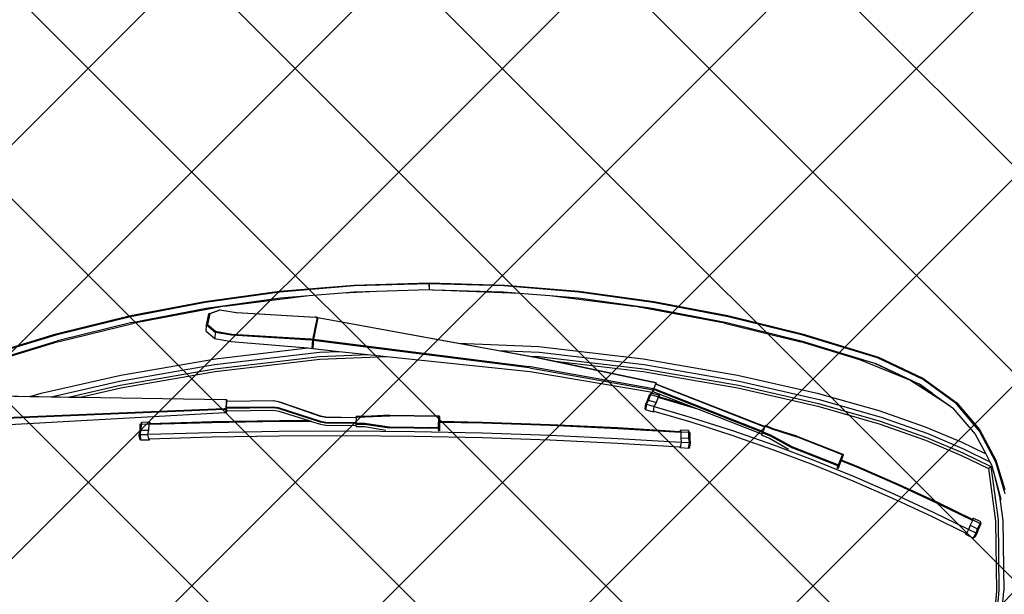
# Model space of a CAD drawing. Units: inches. Extents: x 2167 to 2589, y 1680 to 2489.
# Tile 26 of 38: x 2356 to 2389, y 1796 to 1815. Entities that reach past the tile are written whole.
import ezdxf

# ---------------------------------------------------------------- set-up
doc = ezdxf.new("R2010")
doc.units = ezdxf.units.IN
doc.header["$MEASUREMENT"] = 0
doc.layers.get('0').update_dxf_attribs({"color": 250})
doc.layers.add('C-PRKG-VEHS', color=8, linetype='Continuous', lineweight=13)
doc.layers.add('L-PVMT-PATT', color=252, linetype='Continuous', lineweight=13)
doc.layers.add('Edges', color=250, linetype='Continuous')

# ---------------------------------------------------------------- blocks, each defined once
blk = doc.blocks.new('Nissan Qashqai pl')
at = {"layer": 'Edges'}
for p, q in [((8.4814, 12.6029), (8.5166, 12.6135)), ((8.5216, 12.6139), (8.4838, 12.6027)), ((8.5538, 12.6111), (8.6387, 12.6123)), ((8.6721, 12.6093), (8.6387, 12.6123)), ((8.4444, 12.5834), (8.4814, 12.6029)), ((8.4838, 12.6027), (8.4462, 12.5833)), ((8.4867, 12.5977), (8.5039, 12.6023)), ((8.4889, 12.5969), (8.5531, 12.6055)), ((8.4914, 12.5942), (8.5544, 12.6026)), ((8.5039, 12.6023), (8.528, 12.6088)), ((8.5216, 12.6068), (8.5039, 12.6023)), ((8.5216, 12.6068), (8.5538, 12.6111)), ((8.5301, 12.609), (8.5216, 12.6068)), ((8.5531, 12.6055), (8.6375, 12.6066)), ((8.5544, 12.6026), (8.6386, 12.6037)), ((8.6375, 12.6066), (8.7481, 12.5968)), ((8.6386, 12.6037), (8.7491, 12.594)), ((8.4499, 12.5782), (8.4737, 12.5908)), ((8.4594, 12.5611), (8.4737, 12.5908)), ((8.468, 12.5648), (8.4831, 12.5957)), ((8.4725, 12.563), (8.4889, 12.5969)), ((8.4737, 12.5908), (8.4831, 12.5957)), ((8.4756, 12.5615), (8.4914, 12.5942)), ((8.4831, 12.5957), (8.4867, 12.5977)), ((8.4914, 12.5942), (8.4889, 12.5969)), ((8.4122, 12.5558), (8.4444, 12.5834)), ((8.4462, 12.5833), (8.4134, 12.5554)), ((8.4183, 12.5508), (8.4499, 12.5782)), ((8.5554, 12.5847), (8.551, 12.5757)), ((8.5529, 12.5751), (8.5572, 12.5841)), ((8.5574, 12.5849), (8.5554, 12.5847)), ((8.5572, 12.5841), (8.5554, 12.5847)), ((8.5639, 12.581), (8.5572, 12.5841)), ((8.5574, 12.5849), (8.5584, 12.5846)), ((8.5582, 12.5845), (8.5574, 12.5849)), ((8.5584, 12.5846), (8.5649, 12.5816)), ((8.5595, 12.572), (8.5639, 12.581)), ((8.5687, 12.5791), (8.5639, 12.581)), ((8.5644, 12.5701), (8.5687, 12.5791)), ((8.5649, 12.5816), (8.5693, 12.5799)), ((8.5687, 12.5791), (8.5693, 12.5799)), ((8.5749, 12.5757), (8.5687, 12.5791)), ((8.5693, 12.5799), (8.5739, 12.5774)), ((8.5739, 12.5774), (8.5749, 12.5757)), ((8.4493, 12.5212), (8.468, 12.5648)), ((8.5527, 12.5749), (8.5323, 12.5332)), ((8.5537, 12.5747), (8.5332, 12.5329)), ((8.5647, 12.57), (8.5441, 12.5279)), ((8.5487, 12.5256), (8.5692, 12.5674)), ((8.5527, 12.5749), (8.551, 12.5757)), ((8.551, 12.5757), (8.5528, 12.5751)), ((8.5528, 12.5751), (8.5527, 12.5749)), ((8.5528, 12.5751), (8.5529, 12.5751)), ((8.5529, 12.5751), (8.5537, 12.5747)), ((8.5537, 12.5747), (8.5595, 12.572)), ((8.5595, 12.572), (8.5644, 12.5701)), ((8.5644, 12.5701), (8.5647, 12.57)), ((8.5647, 12.57), (8.5692, 12.5675)), ((8.5692, 12.5674), (8.5692, 12.5675)), ((8.5692, 12.5675), (8.5705, 12.5668)), ((8.5705, 12.5668), (8.5692, 12.5674)), ((8.5749, 12.5757), (8.5705, 12.5668)), ((8.3826, 12.5151), (8.4122, 12.5558)), ((8.4134, 12.5554), (8.3844, 12.5157)), ((8.4411, 12.5178), (8.4594, 12.5611)), ((8.454, 12.5196), (8.4725, 12.563)), ((8.4571, 12.5184), (8.4756, 12.5615)), ((8.4154, 12.5468), (8.3852, 12.4994)), ((8.3901, 12.5113), (8.4154, 12.5468)), ((8.4011, 12.5269), (8.4154, 12.5468)), ((8.4156, 12.547), (8.4154, 12.5468)), ((8.4156, 12.547), (8.4183, 12.5508)), ((8.5323, 12.5332), (8.5103, 12.4859)), ((8.5332, 12.5329), (8.5112, 12.4856)), ((8.4011, 12.5269), (8.3901, 12.5113)), ((8.3904, 12.512), (8.4011, 12.5269)), ((8.4217, 12.4622), (8.4411, 12.5178)), ((8.4296, 12.4651), (8.4493, 12.5212)), ((8.4343, 12.4637), (8.454, 12.5196)), ((8.4375, 12.4627), (8.4571, 12.5184)), ((8.5441, 12.5279), (8.5222, 12.4807)), ((8.5269, 12.4785), (8.5487, 12.5256)), ((8.3573, 12.4618), (8.3826, 12.5151)), ((8.3844, 12.5157), (8.3582, 12.4606)), ((8.3646, 12.4572), (8.39, 12.5111)), ((8.3648, 12.4579), (8.39, 12.5111)), ((8.39, 12.5111), (8.3852, 12.4994)), ((8.39, 12.5111), (8.3901, 12.5113)), ((8.3901, 12.5113), (8.3904, 12.512)), ((8.3852, 12.4994), (8.3608, 12.4393)), ((8.5103, 12.4859), (8.4895, 12.4381)), ((8.5112, 12.4856), (8.4904, 12.4377)), ((8.5222, 12.4807), (8.5014, 12.4329)), ((8.5062, 12.431), (8.5269, 12.4785)), ((8.3296, 12.3703), (8.3573, 12.4618)), ((8.3582, 12.4606), (8.3311, 12.3708)), ((8.3646, 12.4572), (8.3648, 12.4579)), ((8.3648, 12.4579), (8.3648, 12.4579)), ((8.4009, 12.3883), (8.4217, 12.4622)), ((8.4084, 12.3907), (8.4296, 12.4651)), ((8.4133, 12.3896), (8.4343, 12.4637)), ((8.4165, 12.3888), (8.4375, 12.4627)), ((8.3377, 12.3689), (8.3646, 12.4572)), ((8.3608, 12.4393), (8.3392, 12.3684)), ((8.3608, 12.4393), (8.3608, 12.4393)), ((8.4895, 12.4381), (8.4811, 12.4174)), ((8.4904, 12.4377), (8.482, 12.4171)), ((8.5014, 12.4329), (8.4817, 12.3847)), ((8.4866, 12.3829), (8.5062, 12.431)), ((8.4526, 12.3639), (8.4742, 12.4188)), ((8.4747, 12.4185), (8.4532, 12.3636)), ((8.4654, 12.3587), (8.4869, 12.4136)), ((8.4881, 12.4131), (8.4666, 12.3582)), ((8.4742, 12.4188), (8.4754, 12.4193)), ((8.4747, 12.4185), (8.4742, 12.4188)), ((8.4754, 12.4193), (8.4747, 12.4185)), ((8.4869, 12.4136), (8.4747, 12.4185)), ((8.4754, 12.4193), (8.4876, 12.4144)), ((8.4791, 12.4183), (8.4754, 12.4193)), ((8.4811, 12.4174), (8.4791, 12.4183)), ((8.482, 12.4171), (8.4811, 12.4174)), ((8.4912, 12.4133), (8.482, 12.4171)), ((8.4869, 12.4136), (8.4876, 12.4144)), ((8.4881, 12.4131), (8.4869, 12.4136)), ((8.4876, 12.4144), (8.4912, 12.4133)), ((8.4876, 12.4144), (8.4881, 12.4131)), ((8.4914, 12.4121), (8.4881, 12.4131)), ((8.4913, 12.4133), (8.4912, 12.4133)), ((8.4913, 12.4132), (8.4913, 12.4133)), ((8.3792, 12.2926), (8.4009, 12.3883)), ((8.3864, 12.2945), (8.4084, 12.3907)), ((8.3913, 12.2935), (8.4133, 12.3896)), ((8.3945, 12.2929), (8.4165, 12.3888)), ((8.4817, 12.3847), (8.4633, 12.3359)), ((8.4683, 12.3345), (8.4866, 12.3829)), ((8.3076, 12.281), (8.3296, 12.3703)), ((8.3311, 12.3708), (8.3089, 12.2811)), ((8.3157, 12.2795), (8.3377, 12.3689)), ((8.3166, 12.2767), (8.3392, 12.3684)), ((8.4526, 12.3639), (8.4434, 12.3353)), ((8.4439, 12.335), (8.4532, 12.3636)), ((8.4509, 12.3322), (8.4654, 12.3587)), ((8.4521, 12.3317), (8.4666, 12.3582)), ((8.4547, 12.3309), (8.4682, 12.3538)), ((8.4434, 12.3353), (8.4397, 12.326)), ((8.4403, 12.3257), (8.4439, 12.335)), ((8.4633, 12.3359), (8.4461, 12.2868)), ((8.4472, 12.3229), (8.4509, 12.3322)), ((8.4484, 12.3224), (8.4521, 12.3317)), ((8.4511, 12.3216), (8.4547, 12.3309)), ((8.4512, 12.2856), (8.4683, 12.3345)), ((8.3894, 12.1944), (8.4409, 12.3255)), ((8.4415, 12.3252), (8.3899, 12.1941)), ((8.3951, 12.192), (8.4467, 12.3231)), ((8.4479, 12.3226), (8.3963, 12.1915)), ((8.4209, 12.2475), (8.4502, 12.3219)), ((8.4403, 12.3257), (8.4397, 12.326)), ((8.4409, 12.3255), (8.4403, 12.3257)), ((8.4415, 12.3252), (8.4409, 12.3255)), ((8.4467, 12.3231), (8.4415, 12.3252)), ((8.4472, 12.3229), (8.4467, 12.3231)), ((8.4479, 12.3226), (8.4472, 12.3229)), ((8.4484, 12.3224), (8.4479, 12.3226)), ((8.4502, 12.3219), (8.4484, 12.3224)), ((8.4511, 12.3216), (8.4502, 12.3219)), ((8.3593, 12.1791), (8.3792, 12.2926)), ((8.3662, 12.1803), (8.3864, 12.2945)), ((8.3713, 12.1796), (8.3913, 12.2935)), ((8.3745, 12.1792), (8.3945, 12.2929)), ((8.2905, 12.1918), (8.3076, 12.281)), ((8.3089, 12.2811), (8.2916, 12.1913)), ((8.4461, 12.2868), (8.4302, 12.2373)), ((8.4353, 12.2363), (8.4512, 12.2856)), ((8.3166, 12.2767), (8.296, 12.168)), ((8.2985, 12.1901), (8.3157, 12.2795)), ((8.4163, 12.2359), (8.4209, 12.2475)), ((8.4209, 12.2475), (8.4191, 12.2418)), ((8.3986, 12.1908), (8.4163, 12.2359)), ((8.4163, 12.2359), (8.4052, 12.1979)), ((8.4191, 12.2418), (8.4061, 12.1973)), ((8.4302, 12.2373), (8.4171, 12.1926)), ((8.4224, 12.1919), (8.4353, 12.2363)), ((8.4457, 12.2337), (8.4452, 12.2238)), ((8.4475, 12.2348), (8.4457, 12.2337)), ((8.4476, 12.2341), (8.4457, 12.2337)), ((8.4471, 12.2242), (8.4476, 12.2341)), ((8.4475, 12.2348), (8.4484, 12.235)), ((8.4555, 12.2348), (8.4475, 12.2348)), ((8.4549, 12.2341), (8.4476, 12.2341)), ((8.4484, 12.235), (8.4557, 12.235)), ((8.4544, 12.2242), (8.4549, 12.2341)), ((8.46, 12.2348), (8.4549, 12.2341)), ((8.4557, 12.235), (8.4603, 12.2357)), ((8.4595, 12.2249), (8.46, 12.2348)), ((8.46, 12.2348), (8.4603, 12.2357)), ((8.4671, 12.2337), (8.46, 12.2348)), ((8.4603, 12.2357), (8.4655, 12.2348)), ((8.4655, 12.2348), (8.4671, 12.2337)), ((8.4671, 12.2337), (8.4666, 12.2237)), ((8.4471, 12.2238), (8.4425, 12.1485)), ((8.448, 12.2241), (8.4435, 12.1487)), ((8.4452, 12.2238), (8.4471, 12.2242)), ((8.4471, 12.2238), (8.4452, 12.2238)), ((8.4471, 12.2242), (8.4544, 12.2242)), ((8.4471, 12.2239), (8.4471, 12.2238)), ((8.4544, 12.2242), (8.4595, 12.2249)), ((8.4601, 12.2247), (8.4555, 12.1488)), ((8.4595, 12.2249), (8.4666, 12.2237)), ((8.4607, 12.1481), (8.4652, 12.2237)), ((8.4652, 12.2237), (8.4652, 12.2238)), ((8.4666, 12.2237), (8.4652, 12.2237)), ((8.4035, 12.1986), (8.4007, 12.189)), ((8.4023, 12.1879), (8.4052, 12.1975)), ((8.4052, 12.1975), (8.4035, 12.1986)), ((8.4035, 12.1986), (8.4052, 12.1979)), ((8.4052, 12.1979), (8.4052, 12.1978)), ((8.412, 12.195), (8.4052, 12.1975)), ((8.2781, 12.1018), (8.2905, 12.1918)), ((8.2916, 12.1913), (8.2793, 12.1016)), ((8.2862, 12.1008), (8.2985, 12.1901)), ((8.3887, 12.1946), (8.3575, 12.0475)), ((8.3882, 12.1948), (8.3618, 12.07)), ((8.3957, 12.1917), (8.3688, 12.0419)), ((8.3702, 12.0427), (8.3969, 12.1913)), ((8.3746, 12.0435), (8.3995, 12.1905)), ((8.3887, 12.1946), (8.3882, 12.1948)), ((8.3882, 12.1948), (8.3894, 12.1944)), ((8.3894, 12.1944), (8.3887, 12.1946)), ((8.3894, 12.1944), (8.3894, 12.1944)), ((8.3894, 12.1944), (8.3899, 12.1941)), ((8.3899, 12.1941), (8.3951, 12.192)), ((8.3951, 12.192), (8.3963, 12.1915)), ((8.3957, 12.1917), (8.3951, 12.192)), ((8.3969, 12.1913), (8.3957, 12.1917)), ((8.3963, 12.1915), (8.3986, 12.1908)), ((8.3995, 12.1905), (8.3969, 12.1913)), ((8.3995, 12.1905), (8.3986, 12.1908)), ((8.4007, 12.189), (8.4023, 12.1879)), ((8.4007, 12.189), (8.402, 12.1874)), ((8.4028, 12.1868), (8.402, 12.1874)), ((8.402, 12.1874), (8.4027, 12.1871)), ((8.4023, 12.1879), (8.4092, 12.1855)), ((8.4097, 12.1844), (8.4028, 12.1868)), ((8.4092, 12.1855), (8.412, 12.195)), ((8.4167, 12.1925), (8.412, 12.195)), ((8.4139, 12.1829), (8.4167, 12.1925)), ((8.4237, 12.1914), (8.4167, 12.1925)), ((8.4237, 12.1914), (8.4209, 12.1819)), ((8.4223, 12.1918), (8.4224, 12.1919)), ((8.4224, 12.1919), (8.4237, 12.1914)), ((8.3448, 12.0536), (8.3593, 12.1791)), ((8.3516, 12.0542), (8.3662, 12.1803)), ((8.3567, 12.0538), (8.3713, 12.1796)), ((8.3618, 12.07), (8.3745, 12.1792)), ((8.4092, 12.1855), (8.4139, 12.1829)), ((8.4139, 12.1821), (8.4097, 12.1844)), ((8.4139, 12.1829), (8.4209, 12.1819)), ((8.4139, 12.1821), (8.4139, 12.1829)), ((8.4191, 12.1813), (8.4139, 12.1821)), ((8.4209, 12.1819), (8.4191, 12.1813)), ((8.2834, 12.0669), (8.296, 12.168)), ((8.4425, 12.1485), (8.4387, 12.0674)), ((8.4435, 12.1487), (8.4397, 12.0674)), ((8.4555, 12.1488), (8.4517, 12.0674)), ((8.4568, 12.0669), (8.4607, 12.1481)), ((8.2708, 12.0123), (8.2781, 12.1018)), ((8.2793, 12.1016), (8.2719, 12.0118)), ((8.2834, 12.0669), (8.2862, 12.1008)), ((8.3618, 12.07), (8.3574, 12.0489)), ((8.4387, 12.0674), (8.4359, 11.9861)), ((8.4397, 12.0674), (8.4369, 11.9861)), ((8.4517, 12.0674), (8.4489, 11.9858)), ((8.2804, 12.0305), (8.2834, 12.0669)), ((8.4541, 11.9857), (8.4568, 12.0669)), ((8.3575, 12.0475), (8.3104, 11.7881)), ((8.3406, 11.9567), (8.3448, 12.0536)), ((8.3495, 12.0053), (8.3516, 12.0542)), ((8.3562, 12.0421), (8.3567, 12.0538)), ((8.3562, 12.0421), (8.3574, 12.0489)), ((8.336, 11.7828), (8.3688, 12.0419)), ((8.3702, 12.0427), (8.3374, 11.7826)), ((8.3495, 12.0053), (8.3562, 12.0421)), ((8.3565, 11.8707), (8.3746, 12.0435)), ((8.2765, 11.9273), (8.2804, 12.0305)), ((8.2788, 12.0114), (8.2804, 12.0305)), ((8.2682, 11.9221), (8.2708, 12.0123)), ((8.2719, 12.0118), (8.2695, 11.9221)), ((8.2765, 11.9273), (8.2788, 12.0114)), ((8.3406, 11.9567), (8.3495, 12.0053)), ((8.4359, 11.9861), (8.4348, 11.9346)), ((8.4369, 11.9861), (8.4358, 11.9346)), ((8.4489, 11.9858), (8.4471, 11.9043)), ((8.4523, 11.9043), (8.4541, 11.9857)), ((8.31, 11.7882), (8.3406, 11.9567)), ((8.2763, 11.9223), (8.2764, 11.9263)), ((8.2764, 11.9263), (8.2765, 11.9273)), ((8.4272, 11.8746), (8.4281, 11.9336)), ((8.4287, 11.9335), (8.4278, 11.8745)), ((8.4281, 11.9336), (8.429, 11.9345)), ((8.4281, 11.9336), (8.4287, 11.9336)), ((8.4287, 11.9335), (8.4281, 11.9336)), ((8.429, 11.9345), (8.4287, 11.9336)), ((8.4287, 11.9336), (8.4287, 11.9335)), ((8.4418, 11.9332), (8.4287, 11.9335)), ((8.4328, 11.9347), (8.429, 11.9345)), ((8.429, 11.9345), (8.4326, 11.9345)), ((8.4328, 11.9347), (8.4326, 11.9345)), ((8.4326, 11.9345), (8.4348, 11.9344)), ((8.4348, 11.9346), (8.4328, 11.9347)), ((8.4348, 11.9346), (8.4348, 11.9344)), ((8.4358, 11.9346), (8.4348, 11.9346)), ((8.4348, 11.9344), (8.4358, 11.9344)), ((8.4358, 11.9346), (8.4358, 11.9344)), ((8.4459, 11.9344), (8.4358, 11.9346)), ((8.4358, 11.9344), (8.4422, 11.9342)), ((8.441, 11.8742), (8.4418, 11.9332)), ((8.4418, 11.9332), (8.4422, 11.9342)), ((8.4431, 11.9332), (8.4418, 11.9332)), ((8.4422, 11.9342), (8.4459, 11.9344)), ((8.4422, 11.9342), (8.4431, 11.9332)), ((8.4431, 11.9332), (8.4422, 11.8742)), ((8.4464, 11.9334), (8.4431, 11.9332)), ((8.4459, 11.9344), (8.4459, 11.9344)), ((8.2708, 11.8319), (8.2682, 11.9221)), ((8.2763, 11.9223), (8.2695, 11.9221)), ((8.2695, 11.9221), (8.2763, 11.9219)), ((8.2695, 11.9221), (8.2719, 11.8323)), ((8.2763, 11.9219), (8.2763, 11.9223)), ((8.2781, 11.8585), (8.2763, 11.9219)), ((8.4471, 11.9043), (8.4464, 11.8227)), ((8.4516, 11.823), (8.4523, 11.9043)), ((8.3542, 11.8485), (8.3565, 11.8707)), ((8.3599, 11.7906), (8.3565, 11.8707)), ((8.4272, 11.8746), (8.4286, 11.8445)), ((8.4292, 11.8445), (8.4278, 11.8745)), ((8.4368, 11.8443), (8.441, 11.8742)), ((8.438, 11.8443), (8.4422, 11.8742)), ((8.4408, 11.8444), (8.4452, 11.8698)), ((8.28, 11.818), (8.2781, 11.8585)), ((8.2788, 11.8327), (8.2781, 11.8585)), ((8.2789, 11.8319), (8.2781, 11.8585)), ((8.3505, 11.8139), (8.3542, 11.8485)), ((8.3567, 11.7903), (8.3542, 11.8485)), ((8.4286, 11.8445), (8.4285, 11.8345)), ((8.4291, 11.8345), (8.4292, 11.8445)), ((8.4366, 11.8345), (8.4368, 11.8443)), ((8.4379, 11.8345), (8.438, 11.8443)), ((8.4406, 11.8344), (8.4408, 11.8444)), ((8.2781, 11.7423), (8.2708, 11.8319)), ((8.2719, 11.8323), (8.2793, 11.7426)), ((8.2789, 11.8319), (8.2788, 11.8327)), ((8.28, 11.818), (8.2789, 11.8319)), ((8.4291, 11.8345), (8.4285, 11.8345)), ((8.4298, 11.8345), (8.4291, 11.8345)), ((8.4292, 11.7978), (8.4298, 11.8345)), ((8.4304, 11.8345), (8.4298, 11.7978)), ((8.4304, 11.8345), (8.4298, 11.8345)), ((8.436, 11.8344), (8.4304, 11.8345)), ((8.4355, 11.7977), (8.436, 11.8344)), ((8.4366, 11.8343), (8.436, 11.8344)), ((8.4366, 11.8345), (8.4379, 11.8345)), ((8.4366, 11.8344), (8.4366, 11.8345)), ((8.4373, 11.8344), (8.4366, 11.8344)), ((8.4373, 11.8344), (8.4366, 11.8343)), ((8.4366, 11.8343), (8.4366, 11.8344)), ((8.4373, 11.8344), (8.4367, 11.7977)), ((8.4379, 11.8344), (8.4373, 11.8344)), ((8.4379, 11.8343), (8.4373, 11.8344)), ((8.4379, 11.8344), (8.4379, 11.8345)), ((8.4397, 11.8344), (8.4379, 11.8343)), ((8.4379, 11.8343), (8.4379, 11.8344)), ((8.4391, 11.7978), (8.4397, 11.8344)), ((8.4406, 11.8344), (8.4397, 11.8344)), ((8.4464, 11.8227), (8.4468, 11.7413)), ((8.452, 11.7418), (8.4516, 11.823)), ((8.2834, 11.7773), (8.28, 11.818)), ((8.3472, 11.7821), (8.3505, 11.8139)), ((8.3516, 11.79), (8.3505, 11.8139)), ((8.4281, 11.7914), (8.4292, 11.7978)), ((8.4298, 11.7978), (8.4287, 11.7914)), ((8.4344, 11.7912), (8.4355, 11.7977)), ((8.4367, 11.7977), (8.4357, 11.7912)), ((8.4381, 11.7914), (8.4391, 11.7978)), ((8.3038, 11.6903), (8.3095, 11.7853)), ((8.3099, 11.7851), (8.3042, 11.6901)), ((8.3092, 11.7863), (8.3093, 11.7873)), ((8.3092, 11.7863), (8.3099, 11.7851)), ((8.3095, 11.7853), (8.3092, 11.7863)), ((8.3093, 11.7873), (8.3367, 11.7816)), ((8.3159, 11.7869), (8.3093, 11.7873)), ((8.31, 11.7882), (8.3104, 11.7881)), ((8.3104, 11.7881), (8.3159, 11.7869)), ((8.3159, 11.7869), (8.336, 11.7828)), ((8.3662, 11.6639), (8.3516, 11.79)), ((8.3713, 11.6645), (8.3567, 11.7903)), ((8.3745, 11.665), (8.3599, 11.7906)), ((8.4107, 11.7411), (8.4281, 11.7914)), ((8.4287, 11.7914), (8.4111, 11.741)), ((8.4179, 11.7406), (8.4344, 11.7912)), ((8.4357, 11.7912), (8.4193, 11.7407)), ((8.4347, 11.7805), (8.4381, 11.7914)), ((8.296, 11.6762), (8.2834, 11.7773)), ((8.2862, 11.7434), (8.2834, 11.7773)), ((8.3298, 11.6848), (8.3355, 11.7798)), ((8.3369, 11.7796), (8.3312, 11.6846)), ((8.3355, 11.7798), (8.3366, 11.7806)), ((8.336, 11.7828), (8.3374, 11.7826)), ((8.3367, 11.7816), (8.3366, 11.7806)), ((8.3366, 11.7806), (8.3369, 11.7796)), ((8.3367, 11.7816), (8.347, 11.7811)), ((8.3374, 11.7826), (8.3406, 11.7824)), ((8.3385, 11.6842), (8.3464, 11.7761)), ((8.3458, 11.7813), (8.3406, 11.7824)), ((8.3406, 11.7824), (8.3457, 11.7821)), ((8.3458, 11.7813), (8.3457, 11.7821)), ((8.3457, 11.7821), (8.3472, 11.7821)), ((8.347, 11.7811), (8.3458, 11.7813)), ((8.3464, 11.7761), (8.3467, 11.7791)), ((8.3593, 11.6651), (8.3464, 11.7761)), ((8.3467, 11.7791), (8.347, 11.7811)), ((8.4222, 11.7413), (8.4337, 11.7775)), ((8.4337, 11.7775), (8.4347, 11.7805)), ((8.4337, 11.7775), (8.4339, 11.7423)), ((8.4347, 11.7805), (8.4348, 11.7421)), ((8.2905, 11.6524), (8.2781, 11.7423)), ((8.2793, 11.7426), (8.2916, 11.6528)), ((8.2985, 11.654), (8.2862, 11.7434)), ((8.4097, 11.7348), (8.4107, 11.7411)), ((8.4111, 11.741), (8.41, 11.7346)), ((8.417, 11.7342), (8.4179, 11.7406)), ((8.4193, 11.7407), (8.4183, 11.7343)), ((8.4213, 11.735), (8.4222, 11.7413)), ((8.4339, 11.7423), (8.4353, 11.6613)), ((8.4348, 11.7421), (8.4362, 11.661)), ((8.4468, 11.7413), (8.4482, 11.66)), ((8.4534, 11.6608), (8.452, 11.7418)), ((8.4104, 11.6791), (8.4097, 11.7348)), ((8.41, 11.7346), (8.4108, 11.6791)), ((8.4177, 11.678), (8.417, 11.7342)), ((8.4183, 11.7343), (8.4191, 11.678)), ((8.4221, 11.6787), (8.4213, 11.735)), ((8.3005, 11.6706), (8.3038, 11.6903)), ((8.3042, 11.6901), (8.3009, 11.6704)), ((8.3264, 11.6652), (8.3298, 11.6848)), ((8.3312, 11.6846), (8.3278, 11.665)), ((8.3352, 11.6646), (8.3385, 11.6842)), ((8.4082, 11.6785), (8.4104, 11.6791)), ((8.4082, 11.6785), (8.4086, 11.6784)), ((8.4082, 11.6766), (8.4082, 11.6785)), ((8.4086, 11.6784), (8.4086, 11.6764)), ((8.4086, 11.6784), (8.4117, 11.6782)), ((8.4104, 11.6791), (8.4108, 11.6791)), ((8.4104, 11.6786), (8.4104, 11.6791)), ((8.4108, 11.6786), (8.4104, 11.6786)), ((8.4104, 11.6786), (8.4108, 11.6784)), ((8.4108, 11.6791), (8.4108, 11.6786)), ((8.4108, 11.6786), (8.4108, 11.6784)), ((8.4108, 11.6784), (8.4117, 11.6783)), ((8.4117, 11.6783), (8.4117, 11.6782)), ((8.4117, 11.6783), (8.4177, 11.678)), ((8.4117, 11.6782), (8.419, 11.6778)), ((8.4177, 11.678), (8.4191, 11.678)), ((8.419, 11.6778), (8.4203, 11.6778)), ((8.419, 11.6758), (8.419, 11.6778)), ((8.4191, 11.678), (8.4221, 11.6787)), ((8.4238, 11.6786), (8.4203, 11.6778)), ((8.4203, 11.6778), (8.4204, 11.6758)), ((8.4238, 11.6786), (8.4221, 11.6787)), ((8.4238, 11.6766), (8.4238, 11.6786)), ((8.296, 11.6762), (8.3166, 11.5675)), ((8.3053, 11.6574), (8.3005, 11.6706)), ((8.3009, 11.6704), (8.3054, 11.6583)), ((8.3182, 11.6557), (8.3264, 11.6652)), ((8.3792, 11.5515), (8.3593, 11.6651)), ((8.4086, 11.6764), (8.4045, 11.4011)), ((8.4056, 11.5028), (8.4082, 11.6766)), ((8.4305, 11.3996), (8.419, 11.6758)), ((8.4204, 11.6758), (8.4319, 11.3996)), ((8.4394, 11.4014), (8.4238, 11.6766)), ((8.3157, 11.5647), (8.2985, 11.654)), ((8.3054, 11.6583), (8.3053, 11.6574)), ((8.319, 11.6546), (8.3053, 11.6574)), ((8.3054, 11.6583), (8.3182, 11.6557)), ((8.319, 11.6546), (8.3182, 11.6557)), ((8.3278, 11.665), (8.319, 11.6546)), ((8.3264, 11.6542), (8.319, 11.6546)), ((8.3264, 11.6542), (8.3352, 11.6646)), ((8.3278, 11.665), (8.3352, 11.6646)), ((8.3864, 11.5497), (8.3662, 11.6639)), ((8.3913, 11.5506), (8.3713, 11.6645)), ((8.3945, 11.5513), (8.3745, 11.665)), ((8.4353, 11.6613), (8.4375, 11.5863)), ((8.4362, 11.661), (8.4385, 11.5858)), ((8.4482, 11.66), (8.4505, 11.5843)), ((8.4557, 11.5855), (8.4534, 11.6608)), ((8.3076, 11.5631), (8.2905, 11.6524)), ((8.2916, 11.6528), (8.3089, 11.5631)), ((8.4377, 11.5857), (8.4357, 11.5864)), ((8.4357, 11.5864), (8.4359, 11.5765)), ((8.4357, 11.5864), (8.4375, 11.5863)), ((8.4375, 11.5863), (8.4375, 11.5862)), ((8.4379, 11.5758), (8.4377, 11.5857)), ((8.445, 11.5853), (8.4377, 11.5857)), ((8.4452, 11.5754), (8.445, 11.5853)), ((8.4503, 11.5841), (8.445, 11.5853)), ((8.4572, 11.5854), (8.4503, 11.5841)), ((8.4505, 11.5742), (8.4503, 11.5841)), ((8.4557, 11.5855), (8.4572, 11.5854)), ((8.4557, 11.5853), (8.4557, 11.5855)), ((8.4572, 11.5854), (8.4574, 11.5755)), ((8.4359, 11.5765), (8.4379, 11.5758)), ((8.4359, 11.5765), (8.4377, 11.5753)), ((8.4387, 11.5749), (8.4377, 11.5753)), ((8.4379, 11.5758), (8.4452, 11.5754)), ((8.4384, 11.5752), (8.4457, 11.5749)), ((8.446, 11.5746), (8.4387, 11.5749)), ((8.4452, 11.5754), (8.4505, 11.5742)), ((8.4507, 11.5734), (8.446, 11.5746)), ((8.4505, 11.5742), (8.4574, 11.5755)), ((8.4507, 11.5734), (8.4505, 11.5742)), ((8.4559, 11.5744), (8.4507, 11.5734)), ((8.4574, 11.5755), (8.4559, 11.5744)), ((8.3296, 11.4739), (8.3076, 11.5631)), ((8.3089, 11.5631), (8.3311, 11.4733)), ((8.3157, 11.5647), (8.3377, 11.4753)), ((8.3392, 11.4758), (8.3166, 11.5675)), ((8.4009, 11.4559), (8.3792, 11.5515)), ((8.4051, 11.4678), (8.3864, 11.5497)), ((8.4054, 11.4887), (8.3913, 11.5506)), ((8.4056, 11.5028), (8.3945, 11.5513)), ((8.4054, 11.4887), (8.4056, 11.5028)), ((8.4051, 11.4678), (8.4054, 11.4887)), ((8.3392, 11.4758), (8.3608, 11.4048)), ((8.3573, 11.3824), (8.3296, 11.4739)), ((8.3311, 11.4733), (8.3582, 11.3836)), ((8.3648, 11.3863), (8.3377, 11.4753)), ((8.4048, 11.4423), (8.4051, 11.4678)), ((8.4048, 11.4423), (8.4009, 11.4559)), ((8.4041, 11.4013), (8.4048, 11.4423))]:
    blk.add_line(p, q, dxfattribs=at)
blk = doc.blocks.new('car')
blk.add_blockref('Nissan Qashqai pl', (-9.7433, -11.9151))
blk = doc.blocks.new('carr')
blk.add_blockref('car', (0.5124, -0.007))

msp = doc.modelspace()

# ---------------------------------------------------------------- hatches: boundary and pattern name
at = {"layer": 'L-PVMT-PATT'}
h = msp.add_hatch(dxfattribs=at)
h.set_pattern_fill('ANSI37', color=256, scale=40)
h.paths.add_polyline_path([(2417.548, 1783.695), (2417.548, 1846.042), (2239.361, 1846.042), (2239.361, 1687.695), (2369.843, 1687.695), (2369.843, 1696.695), (2375.607, 1696.695), (2416.107, 1696.695), (2417.548, 1696.695)])

# ---------------------------------------------------------------- block references
at = {"layer": 'C-PRKG-VEHS', "xscale": 28.42784210623918, "yscale": 28.42784210623918, "zscale": 28.42784210623918, "rotation": 270}
msp.add_blockref('carr', (2369.852, 1779.037), dxfattribs=at)

doc.saveas('drawing.dxf')
